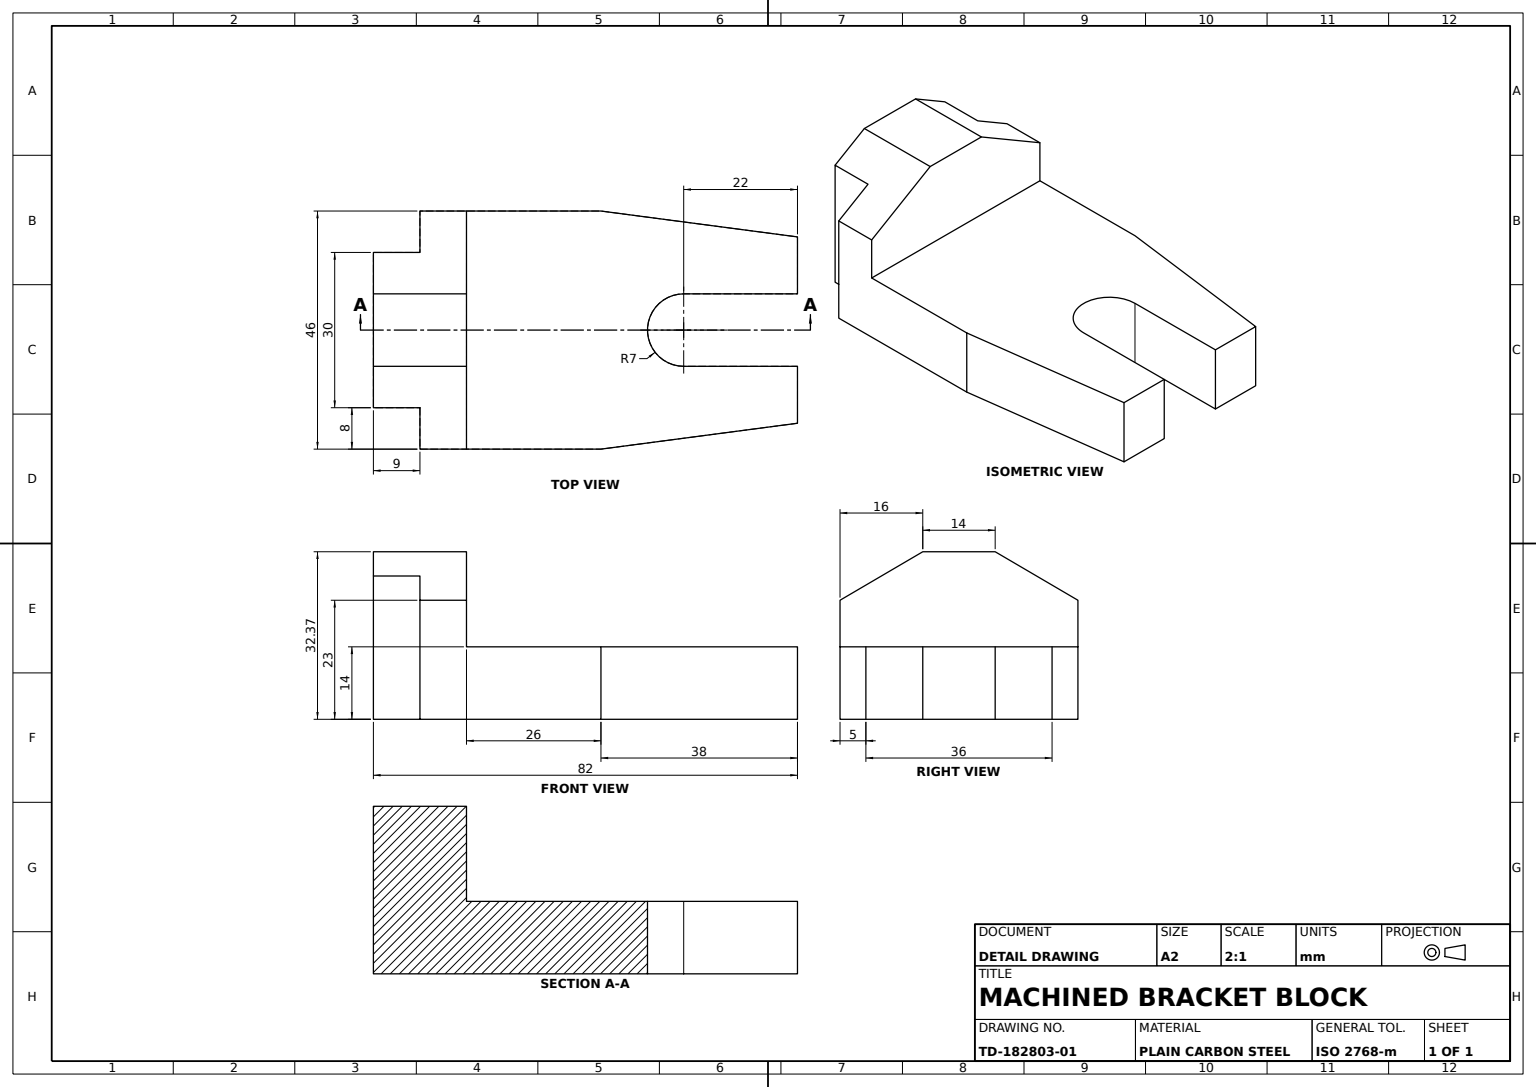
from build123d import *

# Parameters (mm, degrees)
SLOTTED_BASE_PLATE_DEPTH = 14
REAR_UPRIGHT_BLOCK_DEPTH = 23
UPPER_STEP_BLOCK_DEPTH   = 9
TOP_BLOCK_DEPTH          = 9


with BuildPart() as part:
    # Slotted Base Plate Sketch → Slotted Base Plate (new body)
    with BuildSketch(Plane(origin=(0, 0, 0), x_dir=(1, 0, 0), z_dir=(0, 1, 0))):
        Polygon((-45.527413465, -5.526673775), (-45.527413465, -13.526673775), (-36.527413465, -13.526673775), (-36.527413465, 32.473326225), (-45.527413465, 32.473326225), (-45.527413465, 24.473326225), (-54.527413465, 24.473326225), (-54.527413465, -5.526673775), align=None)
        with BuildLine():
            ThreePointArc((5.472586535, 16.473326225), (-1.527413465, 9.473326225), (5.472586535, 2.473326225))
            Line((5.472586535, 2.473326225), (27.472586535, 2.473326225))
            Line((27.472586535, 2.473326225), (27.472586535, -8.526673775))
            Line((27.472586535, -8.526673775), (-10.527413465, -13.526673775))
            Line((-10.527413465, -13.526673775), (-36.527413465, -13.526673775))
            Line((-36.527413465, -13.526673775), (-36.527413465, 32.473326225))
            Line((-36.527413465, 32.473326225), (-10.527413465, 32.473326225))
            Line((-10.527413465, 32.473326225), (27.472586535, 27.473326225))
            Line((27.472586535, 27.473326225), (27.472586535, 16.473326225))
            Line((27.472586535, 16.473326225), (5.472586535, 16.473326225))
        make_face()
    extrude(amount=SLOTTED_BASE_PLATE_DEPTH)

    # Rear Upright Block Sketch → Rear Upright Block (add)
    with BuildSketch(Plane(origin=(0, 0, 0), x_dir=(1, 0, 0), z_dir=(0, 1, 0))):
        Polygon((-45.527413465, 32.473326225), (-36.527413465, 32.473326225), (-36.527413465, -13.526673775), (-45.527413465, -13.526673775), (-45.527413465, -5.526673775), (-54.527413465, -5.526673775), (-54.527413465, 24.473326225), (-45.527413465, 24.473326225), align=None)
    extrude(amount=REAR_UPRIGHT_BLOCK_DEPTH)

    # Upper Step Sketch → Upper Step Block (add)
    with BuildSketch(Plane(origin=(-36.527413465, 0, 0), x_dir=(0, 0, -1), z_dir=(1, 0, 0))):
        Polygon((-13.526673775, 23), (32.473326225, 23), (16.473326225, 32.368724422), (2.473326225, 32.368724422), align=None)
    extrude(amount=-UPPER_STEP_BLOCK_DEPTH)

    # Top Block Sketch → Top Block (add)
    with BuildSketch(Plane.ZY.offset(45.527413465)):
        Polygon((-24.473326225, 23), (-24.473326225, 27.684362211), (-16.473326225, 32.368724422), (-2.473326225, 32.368724422), (5.526673775, 27.684362211), (5.526673775, 23), align=None)
    extrude(amount=TOP_BLOCK_DEPTH)


solid = part.part
